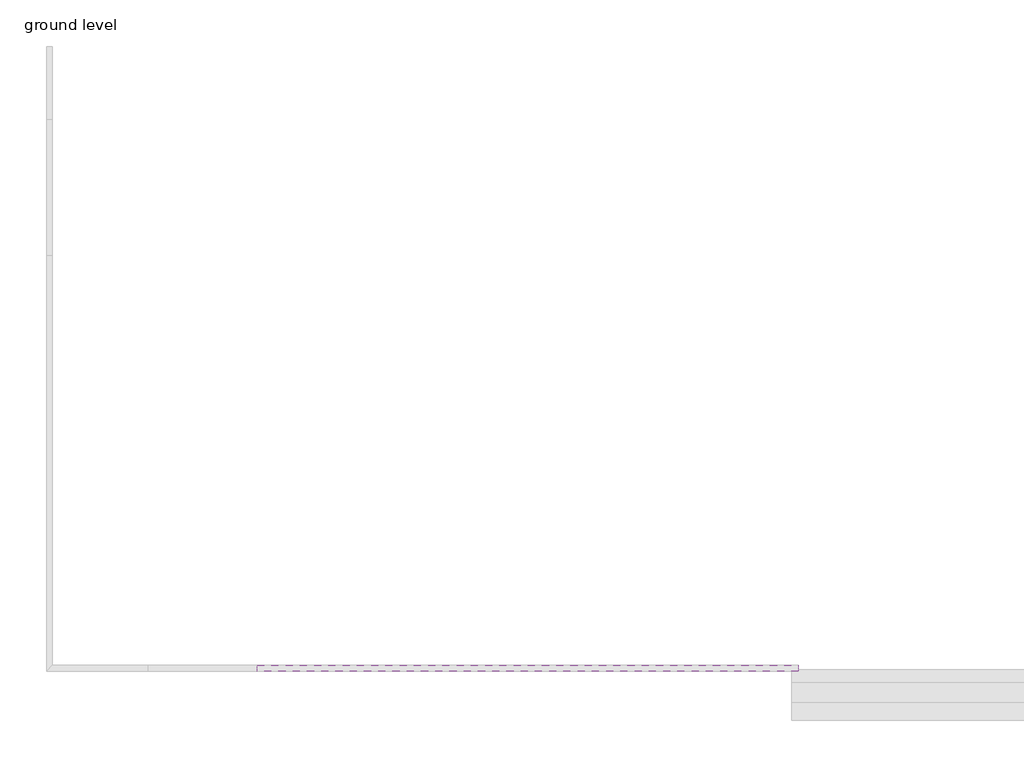
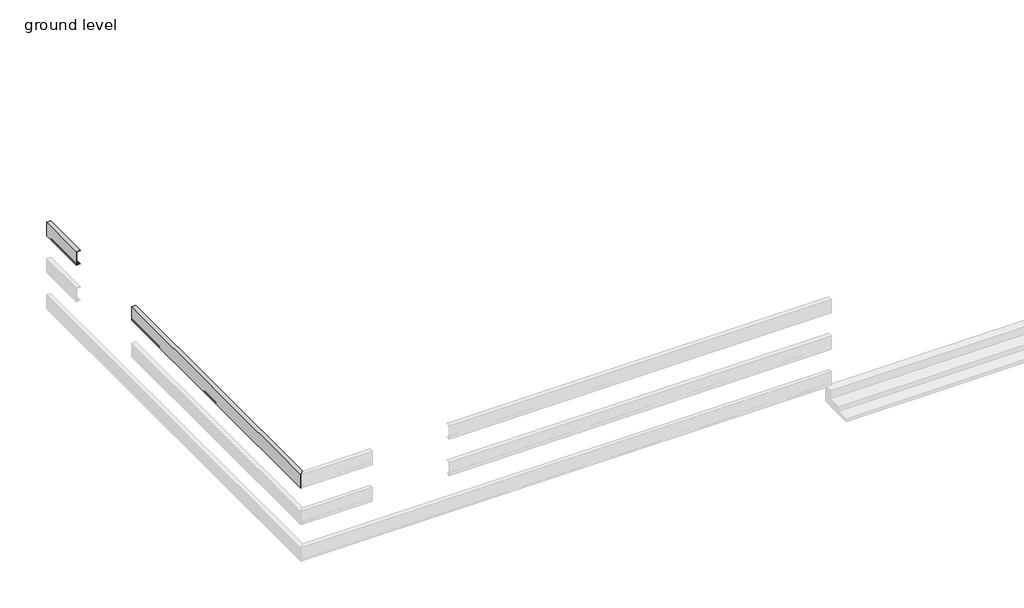
# One storey, part 2 of 3: 1 proxy.
"""IFC4 building model written with IfcOpenShell, lengths in millimetres."""

from ifc_helpers import new_model, si_unit, frame, origin, place, context, project, spatial, polyline, circle_curve, ellipse_curve, element, save
from ifc_brep_helpers import plane_surface, cylinder_surface, revolved_surface, advanced_brep

model = new_model("IFC4")

# Units and contexts
model_context = context("Model", 3, world=origin())
ifc_project = project(units=[si_unit("LENGTHUNIT", "METRE", prefix="MILLI")], contexts=[model_context])

# Site, building, storey
site = spatial("IfcSite", under=ifc_project)
building = spatial("IfcBuilding", under=site)
storey = spatial("IfcBuildingStorey", under=building, Name="ground level", Elevation=0.0)

# Proxy
placement = place(None, origin())
element("IfcBuildingElementProxy", 1, Name="Reveal", ObjectType="Reveal", at=placement, inside=storey, context=model_context, shape_type="AdvancedBrep", body=[
    advanced_brep(
    [(-10842.2672301, -7280.1146427, 1689.1), (-10842.2672301, -7216.8686427, 1689.1), (-10842.2672301, -7216.8686427, 1687.7203242), (-10842.2672301, -7221.2514519, 1682.5465897), (-10842.2672301, -7244.8721427, 1678.6098), (-10842.2672301, -7264.1100243, 1675.40348), (-10842.2672301, -7272.8756427, 1665.056011), (-10842.2672301, -7272.8756427, 1484.543989), (-10842.2672301, -7264.1100243, 1474.19652), (-10842.2672301, -7244.8721427, 1470.9902), (-10842.2672301, -7221.2514519, 1467.0534103), (-10842.2672301, -7216.8686427, 1461.8796758), (-10842.2672301, -7216.8686427, 1460.5), (-10842.2672301, -7280.1146427, 1460.5), (-4797.0672301, -7280.1146427, 1689.1), (-4797.0672301, -7280.1146427, 1460.5), (-4797.0672301, -7216.8686427, 1460.5), (-4797.0672301, -7216.8686427, 1461.8796758), (-4797.0672301, -7221.2514519, 1467.0534103), (-4797.0672301, -7244.8721427, 1470.9902), (-4797.0672301, -7264.1100243, 1474.19652), (-4797.0672301, -7272.8756427, 1484.543989), (-4797.0672301, -7272.8756427, 1665.056011), (-4797.0672301, -7264.1100243, 1675.40348), (-4797.0672301, -7244.8721427, 1678.6098), (-4797.0672301, -7221.2514519, 1682.5465897), (-4797.0672301, -7216.8686427, 1687.7203242), (-4797.0672301, -7216.8686427, 1689.1)],
    [
        (0, 1),
        (1, 2),
        (2, 3, circle_curve(frame((-10842.2672301, -7222.1137427, 1687.7203242), z_axis=(-1.0, 0.0, 0.0), x_axis=(0.0, 1.0, 0.0)), 5.2451)),
        (3, 4),
        (4, 5),
        (5, 6, circle_curve(frame((-10842.2672301, -7262.3854427, 1665.056011), z_axis=(1.0, 0.0, 0.0), x_axis=(0.0, 1.0, 0.0)), 10.4902)),
        (6, 7),
        (7, 8, circle_curve(frame((-10842.2672301, -7262.3854427, 1484.543989), z_axis=(1.0, 0.0, 0.0), x_axis=(0.0, 1.0, 0.0)), 10.4902)),
        (8, 9),
        (9, 10),
        (10, 11, circle_curve(frame((-10842.2672301, -7222.1137427, 1461.8796758), z_axis=(-1.0, 0.0, 0.0), x_axis=(0.0, 1.0, 0.0)), 5.2451)),
        (11, 12),
        (12, 13),
        (13, 0),
        (14, 15),
        (15, 16),
        (16, 17),
        (17, 18, circle_curve(frame((-4797.0672301, -7222.1137427, 1461.8796758), z_axis=(1.0, 0.0, 0.0), x_axis=(0.0, 1.0, 0.0)), 5.2451)),
        (18, 19),
        (19, 20),
        (20, 21, circle_curve(frame((-4797.0672301, -7262.3854427, 1484.543989), z_axis=(-1.0, 0.0, 0.0), x_axis=(0.0, 1.0, 0.0)), 10.4902)),
        (21, 22),
        (22, 23, circle_curve(frame((-4797.0672301, -7262.3854427, 1665.056011), z_axis=(-1.0, 0.0, 0.0), x_axis=(0.0, 1.0, 0.0)), 10.4902)),
        (23, 24),
        (24, 25),
        (25, 26, circle_curve(frame((-4797.0672301, -7222.1137427, 1687.7203242), z_axis=(1.0, 0.0, 0.0), x_axis=(0.0, 1.0, 0.0)), 5.2451)),
        (26, 27),
        (27, 14),
        (0, 14),
        (27, 1),
        (26, 2),
        (25, 3),
        (24, 4),
        (23, 5),
        (22, 6),
        (21, 7),
        (20, 8),
        (19, 9),
        (18, 10),
        (17, 11),
        (16, 12),
        (15, 13),
    ],
    [
        plane_surface(frame((-10842.2672301, -7036.6302427, 914.4), z_axis=(-1.0, 0.0, 0.0), x_axis=(0.0, -1.0, 0.0))),
        plane_surface(frame((-4797.0672301, -7265.2302427, 1450.6898298), z_axis=(1.0, 0.0, 0.0), x_axis=(0.0, 1.0, 0.0))),
        plane_surface(frame((-10842.2672301, -7280.1146427, 1689.1), z_axis=(0.0, 0.0, 1.0), x_axis=(1.0, 0.0, 0.0))),
        plane_surface(frame((-10842.2672301, -7216.8686427, 1689.1), z_axis=(0.0, 1.0, 0.0), x_axis=(1.0, 0.0, 0.0))),
        cylinder_surface(frame((-10842.2672301, -7222.1137427, 1687.7203242), z_axis=(-1.0, 0.0, 0.0), x_axis=(0.0, 1.0, 0.0)), 5.2451),
        plane_surface(frame((-10842.2672301, -7221.2514519, 1682.5465897), z_axis=(0.0, 0.16439930721687082, -0.9863938705135049), x_axis=(1.0, 0.0, 0.0))),
        plane_surface(frame((-10842.2672301, -7244.8721427, 1678.6098), z_axis=(0.0, 0.16439930721687146, -0.9863938705135048), x_axis=(1.0, 0.0, 0.0))),
        revolved_surface(polyline([(-4797.0672301, -7251.8952426999995, 1665.056011), (-10842.2672301, -7251.8952426999995, 1665.056011)]), (-10842.2672301, -7262.3854427, 1665.056011), (1.0, 0.0, 0.0)),
        plane_surface(frame((-10842.2672301, -7272.8756427, 1665.056011), z_axis=(0.0, 1.0, 0.0), x_axis=(1.0, 0.0, 0.0))),
        revolved_surface(polyline([(-4797.0672301, -7251.8952426999995, 1484.543989), (-10842.2672301, -7251.8952426999995, 1484.543989)]), (-10842.2672301, -7262.3854427, 1484.543989), (1.0, 0.0, 0.0)),
        plane_surface(frame((-10842.2672301, -7264.1100243, 1474.19652), z_axis=(0.0, 0.1643993072168769, 0.9863938705135039), x_axis=(1.0, 0.0, 0.0))),
        plane_surface(frame((-10842.2672301, -7244.8721427, 1470.9902), z_axis=(0.0, 0.16439930721687793, 0.9863938705135037), x_axis=(1.0, 0.0, 0.0))),
        cylinder_surface(frame((-10842.2672301, -7222.1137427, 1461.8796758), z_axis=(-1.0, 0.0, 0.0), x_axis=(0.0, 1.0, 0.0)), 5.2451),
        plane_surface(frame((-10842.2672301, -7216.8686427, 1461.8796758), z_axis=(0.0, 1.0, 0.0), x_axis=(1.0, 0.0, 0.0))),
        plane_surface(frame((-10842.2672301, -7216.8686427, 1460.5), z_axis=(0.0, 0.0, -1.0), x_axis=(1.0, 0.0, 0.0))),
        plane_surface(frame((-10842.2672301, -7280.1146427, 1460.5), z_axis=(0.0, -1.0, 0.0), x_axis=(1.0, 0.0, 0.0))),
    ],
    [
        (0, [[1, 2, 3, 4, 5, 6, 7, 8, 9, 10, 11, 12, 13, 14]]),
        (1, [[15, 16, 17, 18, 19, 20, 21, 22, 23, 24, 25, 26, 27, 28]]),
        (2, [[-1, 29, -28, 30]]),
        (3, [[-2, -30, -27, 31]]),
        (4, [[-3, -31, -26, 32]]),
        (5, [[-4, -32, -25, 33]]),
        (6, [[-5, -33, -24, 34]]),
        (7, [[-6, -34, -23, 35]]),
        (8, [[-7, -35, -22, 36]]),
        (9, [[-8, -36, -21, 37]]),
        (10, [[-9, -37, -20, 38]]),
        (11, [[-10, -38, -19, 39]]),
        (12, [[-11, -39, -18, 40]]),
        (13, [[-12, -40, -17, 41]]),
        (14, [[-13, -41, -16, 42]]),
        (15, [[-14, -42, -15, -29]]),
    ],
),
    advanced_brep(
    [(-13193.9516301, -7280.1146427, 1689.1), (-13130.7056301, -7216.8686427, 1689.1), (-13130.7056301, -7216.8686427, 1687.7203242), (-13135.0884393, -7221.2514519, 1682.5465897), (-13158.7091301, -7244.8721427, 1678.6098), (-13177.9470117, -7264.1100243, 1675.40348), (-13186.7126301, -7272.8756427, 1665.056011), (-13186.7126301, -7272.8756427, 1484.543989), (-13177.9470117, -7264.1100243, 1474.19652), (-13158.7091301, -7244.8721427, 1470.9902), (-13135.0884393, -7221.2514519, 1467.0534103), (-13130.7056301, -7216.8686427, 1461.8796758), (-13130.7056301, -7216.8686427, 1460.5), (-13193.9516301, -7280.1146427, 1460.5), (-12061.4672301, -7280.1146427, 1689.1), (-12061.4672301, -7280.1146427, 1460.5), (-12061.4672301, -7216.8686427, 1460.5), (-12061.4672301, -7216.8686427, 1461.8796758), (-12061.4672301, -7221.2514519, 1467.0534103), (-12061.4672301, -7244.8721427, 1470.9902), (-12061.4672301, -7264.1100243, 1474.19652), (-12061.4672301, -7272.8756427, 1484.543989), (-12061.4672301, -7272.8756427, 1665.056011), (-12061.4672301, -7264.1100243, 1675.40348), (-12061.4672301, -7244.8721427, 1678.6098), (-12061.4672301, -7221.2514519, 1682.5465897), (-12061.4672301, -7216.8686427, 1687.7203242), (-12061.4672301, -7216.8686427, 1689.1)],
    [
        (0, 1),
        (1, 2),
        (2, 3, ellipse_curve(frame((-13135.9507301, -7222.1137427, 1687.7203242), z_axis=(-0.7071067811865476, 0.7071067811865476, 0.0), x_axis=(-0.7071067811865475, -0.7071067811865476, 0.0)), 7.4176916, 5.2451)),
        (3, 4),
        (4, 5),
        (5, 6, ellipse_curve(frame((-13176.2224301, -7262.3854427, 1665.056011), z_axis=(0.7071067811865476, -0.7071067811865476, 0.0), x_axis=(0.7071067811865475, 0.7071067811865476, 0.0)), 14.8353831, 10.4902)),
        (6, 7),
        (7, 8, ellipse_curve(frame((-13176.2224301, -7262.3854427, 1484.543989), z_axis=(0.7071067811865476, -0.7071067811865476, 0.0), x_axis=(0.7071067811865475, 0.7071067811865476, 0.0)), 14.8353831, 10.4902)),
        (8, 9),
        (9, 10),
        (10, 11, ellipse_curve(frame((-13135.9507301, -7222.1137427, 1461.8796758), z_axis=(-0.7071067811865476, 0.7071067811865476, 0.0), x_axis=(-0.7071067811865475, -0.7071067811865476, 0.0)), 7.4176916, 5.2451)),
        (11, 12),
        (12, 13),
        (13, 0),
        (14, 15),
        (15, 16),
        (16, 17),
        (17, 18, circle_curve(frame((-12061.4672301, -7222.1137427, 1461.8796758), z_axis=(1.0, 0.0, 0.0), x_axis=(0.0, 1.0, 0.0)), 5.2451)),
        (18, 19),
        (19, 20),
        (20, 21, circle_curve(frame((-12061.4672301, -7262.3854427, 1484.543989), z_axis=(-1.0, 0.0, 0.0), x_axis=(0.0, 1.0, 0.0)), 10.4902)),
        (21, 22),
        (22, 23, circle_curve(frame((-12061.4672301, -7262.3854427, 1665.056011), z_axis=(-1.0, 0.0, 0.0), x_axis=(0.0, 1.0, 0.0)), 10.4902)),
        (23, 24),
        (24, 25),
        (25, 26, circle_curve(frame((-12061.4672301, -7222.1137427, 1687.7203242), z_axis=(1.0, 0.0, 0.0), x_axis=(0.0, 1.0, 0.0)), 5.2451)),
        (26, 27),
        (27, 14),
        (0, 14),
        (27, 1),
        (26, 2),
        (25, 3),
        (24, 4),
        (23, 5),
        (22, 6),
        (21, 7),
        (20, 8),
        (19, 9),
        (18, 10),
        (17, 11),
        (16, 12),
        (15, 13),
    ],
    [
        plane_surface(frame((-13179.0672301, -7265.2302427, 1270.0), z_axis=(-0.7071067811865476, 0.7071067811865476, 0.0), x_axis=(0.7071067811865476, 0.7071067811865476, 0.0))),
        plane_surface(frame((-12061.4672301, -7036.6302427, 2184.4), z_axis=(1.0, 0.0, 0.0), x_axis=(0.0, -1.0, 0.0))),
        plane_surface(frame((-13193.9516301, -7280.1146427, 1689.1), z_axis=(0.0, 0.0, 1.0), x_axis=(1.0, 0.0, 0.0))),
        plane_surface(frame((-13130.7056301, -7216.8686427, 1689.1), z_axis=(0.0, 1.0, 0.0), x_axis=(1.0, 0.0, 0.0))),
        cylinder_surface(frame((-13179.0672301, -7222.1137427, 1687.7203242), z_axis=(-1.0, 0.0, 0.0), x_axis=(0.0, 1.0, 0.0)), 5.2451),
        plane_surface(frame((-13135.0884393, -7221.2514519, 1682.5465897), z_axis=(0.0, 0.16439930721687082, -0.9863938705135049), x_axis=(1.0, 0.0, 0.0))),
        plane_surface(frame((-13158.7091301, -7244.8721427, 1678.6098), z_axis=(0.0, 0.16439930721687146, -0.9863938705135048), x_axis=(1.0, 0.0, 0.0))),
        revolved_surface(polyline([(-12061.4672301, -7251.8952426999995, 1665.056011), (-13186.7126301, -7251.8952426999995, 1665.056011)]), (-13179.0672301, -7262.3854427, 1665.056011), (1.0, 0.0, 0.0)),
        plane_surface(frame((-13186.7126301, -7272.8756427, 1665.056011), z_axis=(0.0, 1.0, 0.0), x_axis=(1.0, 0.0, 0.0))),
        revolved_surface(polyline([(-12061.4672301, -7251.8952426999995, 1484.543989), (-13186.7126301, -7251.8952426999995, 1484.543989)]), (-13179.0672301, -7262.3854427, 1484.543989), (1.0, 0.0, 0.0)),
        plane_surface(frame((-13177.9470117, -7264.1100243, 1474.19652), z_axis=(0.0, 0.1643993072168769, 0.9863938705135039), x_axis=(1.0, 0.0, 0.0))),
        plane_surface(frame((-13158.7091301, -7244.8721427, 1470.9902), z_axis=(0.0, 0.16439930721687793, 0.9863938705135037), x_axis=(1.0, 0.0, 0.0))),
        cylinder_surface(frame((-13179.0672301, -7222.1137427, 1461.8796758), z_axis=(-1.0, 0.0, 0.0), x_axis=(0.0, 1.0, 0.0)), 5.2451),
        plane_surface(frame((-13130.7056301, -7216.8686427, 1461.8796758), z_axis=(0.0, 1.0, 0.0), x_axis=(1.0, 0.0, 0.0))),
        plane_surface(frame((-13130.7056301, -7216.8686427, 1460.5), z_axis=(0.0, 0.0, -1.0), x_axis=(1.0, 0.0, 0.0))),
        plane_surface(frame((-13193.9516301, -7280.1146427, 1460.5), z_axis=(0.0, -1.0, 0.0), x_axis=(1.0, 0.0, 0.0))),
    ],
    [
        (0, [[1, 2, 3, 4, 5, 6, 7, 8, 9, 10, 11, 12, 13, 14]]),
        (1, [[15, 16, 17, 18, 19, 20, 21, 22, 23, 24, 25, 26, 27, 28]]),
        (2, [[-1, 29, -28, 30]]),
        (3, [[-2, -30, -27, 31]]),
        (4, [[-3, -31, -26, 32]]),
        (5, [[-4, -32, -25, 33]]),
        (6, [[-5, -33, -24, 34]]),
        (7, [[-6, -34, -23, 35]]),
        (8, [[-7, -35, -22, 36]]),
        (9, [[-8, -36, -21, 37]]),
        (10, [[-9, -37, -20, 38]]),
        (11, [[-10, -38, -19, 39]]),
        (12, [[-11, -39, -18, 40]]),
        (13, [[-12, -40, -17, 41]]),
        (14, [[-13, -41, -16, 42]]),
        (15, [[-14, -42, -15, -29]]),
    ],
),
    advanced_brep(
    [(-13193.9516301, -2642.4302427, 1689.1), (-13130.7056301, -2642.4302427, 1689.1), (-13130.7056301, -2642.4302427, 1687.7203242), (-13135.0884393, -2642.4302427, 1682.5465897), (-13158.7091301, -2642.4302427, 1678.6098), (-13177.9470117, -2642.4302427, 1675.40348), (-13186.7126301, -2642.4302427, 1665.056011), (-13186.7126301, -2642.4302427, 1484.543989), (-13177.9470117, -2642.4302427, 1474.19652), (-13158.7091301, -2642.4302427, 1470.9902), (-13135.0884393, -2642.4302427, 1467.0534103), (-13130.7056301, -2642.4302427, 1461.8796758), (-13130.7056301, -2642.4302427, 1460.5), (-13193.9516301, -2642.4302427, 1460.5), (-13193.9516301, -7280.1146427, 1689.1), (-13193.9516301, -7280.1146427, 1460.5), (-13130.7056301, -7216.8686427, 1460.5), (-13130.7056301, -7216.8686427, 1461.8796758), (-13135.0884393, -7221.2514519, 1467.0534103), (-13158.7091301, -7244.8721427, 1470.9902), (-13177.9470117, -7264.1100243, 1474.19652), (-13186.7126301, -7272.8756427, 1484.543989), (-13186.7126301, -7272.8756427, 1665.056011), (-13177.9470117, -7264.1100243, 1675.40348), (-13158.7091301, -7244.8721427, 1678.6098), (-13135.0884393, -7221.2514519, 1682.5465897), (-13130.7056301, -7216.8686427, 1687.7203242), (-13130.7056301, -7216.8686427, 1689.1)],
    [
        (0, 1),
        (1, 2),
        (2, 3, circle_curve(frame((-13135.9507301, -2642.4302427, 1687.7203242), z_axis=(0.0, 1.0, 0.0), x_axis=(1.0, 0.0, 0.0)), 5.2451)),
        (3, 4),
        (4, 5),
        (5, 6, circle_curve(frame((-13176.2224301, -2642.4302427, 1665.056011), z_axis=(0.0, -1.0, 0.0), x_axis=(1.0, 0.0, 0.0)), 10.4902)),
        (6, 7),
        (7, 8, circle_curve(frame((-13176.2224301, -2642.4302427, 1484.543989), z_axis=(0.0, -1.0, 0.0), x_axis=(1.0, 0.0, 0.0)), 10.4902)),
        (8, 9),
        (9, 10),
        (10, 11, circle_curve(frame((-13135.9507301, -2642.4302427, 1461.8796758), z_axis=(0.0, 1.0, 0.0), x_axis=(1.0, 0.0, 0.0)), 5.2451)),
        (11, 12),
        (12, 13),
        (13, 0),
        (14, 15),
        (15, 16),
        (16, 17),
        (17, 18, ellipse_curve(frame((-13135.9507301, -7222.1137427, 1461.8796758), z_axis=(0.7071067811865476, -0.7071067811865476, 0.0), x_axis=(0.7071067811865477, 0.7071067811865474, 0.0)), 7.4176916, 5.2451)),
        (18, 19),
        (19, 20),
        (20, 21, ellipse_curve(frame((-13176.2224301, -7262.3854427, 1484.543989), z_axis=(-0.7071067811865476, 0.7071067811865476, 0.0), x_axis=(-0.7071067811865477, -0.7071067811865474, 0.0)), 14.8353831, 10.4902)),
        (21, 22),
        (22, 23, ellipse_curve(frame((-13176.2224301, -7262.3854427, 1665.056011), z_axis=(-0.7071067811865476, 0.7071067811865476, 0.0), x_axis=(-0.7071067811865477, -0.7071067811865474, 0.0)), 14.8353831, 10.4902)),
        (23, 24),
        (24, 25),
        (25, 26, ellipse_curve(frame((-13135.9507301, -7222.1137427, 1687.7203242), z_axis=(0.7071067811865476, -0.7071067811865476, 0.0), x_axis=(0.7071067811865477, 0.7071067811865474, 0.0)), 7.4176916, 5.2451)),
        (26, 27),
        (27, 14),
        (0, 14),
        (27, 1),
        (26, 2),
        (25, 3),
        (24, 4),
        (23, 5),
        (22, 6),
        (21, 7),
        (20, 8),
        (19, 9),
        (18, 10),
        (17, 11),
        (16, 12),
        (15, 13),
    ],
    [
        plane_surface(frame((-12950.4672301, -2642.4302427, 914.4), z_axis=(0.0, 1.0, 0.0), x_axis=(-1.0, 0.0, 0.0))),
        plane_surface(frame((-13179.0672301, -7265.2302427, 1270.0), z_axis=(0.7071067811865476, -0.7071067811865476, 0.0), x_axis=(0.7071067811865476, 0.7071067811865476, 0.0))),
        plane_surface(frame((-13193.9516301, -2642.4302427, 1689.1), z_axis=(0.0, 0.0, 1.0), x_axis=(0.0, -1.0, 0.0))),
        plane_surface(frame((-13130.7056301, -2642.4302427, 1689.1), z_axis=(1.0, 0.0, 0.0), x_axis=(0.0, -1.0, 0.0))),
        cylinder_surface(frame((-13135.9507301, -2642.4302427, 1687.7203242), z_axis=(0.0, 1.0, 0.0), x_axis=(1.0, 0.0, 0.0)), 5.2451),
        plane_surface(frame((-13135.0884393, -2642.4302427, 1682.5465897), z_axis=(0.16439930721687082, 0.0, -0.9863938705135049), x_axis=(0.0, -1.0, 0.0))),
        plane_surface(frame((-13158.7091301, -2642.4302427, 1678.6098), z_axis=(0.16439930721687146, 0.0, -0.9863938705135048), x_axis=(0.0, -1.0, 0.0))),
        revolved_surface(polyline([(-13165.7322301, -7272.875642700001, 1665.056011), (-13165.7322301, -2642.4302427, 1665.056011)]), (-13176.2224301, -2642.4302427, 1665.056011), (0.0, -1.0, 0.0)),
        plane_surface(frame((-13186.7126301, -2642.4302427, 1665.056011), z_axis=(1.0, 0.0, 0.0), x_axis=(0.0, -1.0, 0.0))),
        revolved_surface(polyline([(-13165.7322301, -7272.875642700001, 1484.543989), (-13165.7322301, -2642.4302427, 1484.543989)]), (-13176.2224301, -2642.4302427, 1484.543989), (0.0, -1.0, 0.0)),
        plane_surface(frame((-13177.9470117, -2642.4302427, 1474.19652), z_axis=(0.1643993072168769, 0.0, 0.9863938705135039), x_axis=(0.0, -1.0, 0.0))),
        plane_surface(frame((-13158.7091301, -2642.4302427, 1470.9902), z_axis=(0.16439930721687793, 0.0, 0.9863938705135037), x_axis=(0.0, -1.0, 0.0))),
        cylinder_surface(frame((-13135.9507301, -2642.4302427, 1461.8796758), z_axis=(0.0, 1.0, 0.0), x_axis=(1.0, 0.0, 0.0)), 5.2451),
        plane_surface(frame((-13130.7056301, -2642.4302427, 1461.8796758), z_axis=(1.0, 0.0, 0.0), x_axis=(0.0, -1.0, 0.0))),
        plane_surface(frame((-13130.7056301, -2642.4302427, 1460.5), z_axis=(0.0, 0.0, -1.0), x_axis=(0.0, -1.0, 0.0))),
        plane_surface(frame((-13193.9516301, -2642.4302427, 1460.5), z_axis=(-1.0, 0.0, 0.0), x_axis=(0.0, -1.0, 0.0))),
    ],
    [
        (0, [[1, 2, 3, 4, 5, 6, 7, 8, 9, 10, 11, 12, 13, 14]]),
        (1, [[15, 16, 17, 18, 19, 20, 21, 22, 23, 24, 25, 26, 27, 28]]),
        (2, [[-1, 29, -28, 30]]),
        (3, [[-2, -30, -27, 31]]),
        (4, [[-3, -31, -26, 32]]),
        (5, [[-4, -32, -25, 33]]),
        (6, [[-5, -33, -24, 34]]),
        (7, [[-6, -34, -23, 35]]),
        (8, [[-7, -35, -22, 36]]),
        (9, [[-8, -36, -21, 37]]),
        (10, [[-9, -37, -20, 38]]),
        (11, [[-10, -38, -19, 39]]),
        (12, [[-11, -39, -18, 40]]),
        (13, [[-12, -40, -17, 41]]),
        (14, [[-13, -41, -16, 42]]),
        (15, [[-14, -42, -15, -29]]),
    ],
),
    advanced_brep(
    [(-13193.9516301, -305.6302427, 1689.1), (-13130.7056301, -305.6302427, 1689.1), (-13130.7056301, -305.6302427, 1687.7203242), (-13135.0884393, -305.6302427, 1682.5465897), (-13158.7091301, -305.6302427, 1678.6098), (-13177.9470117, -305.6302427, 1675.40348), (-13186.7126301, -305.6302427, 1665.056011), (-13186.7126301, -305.6302427, 1484.543989), (-13177.9470117, -305.6302427, 1474.19652), (-13158.7091301, -305.6302427, 1470.9902), (-13135.0884393, -305.6302427, 1467.0534103), (-13130.7056301, -305.6302427, 1461.8796758), (-13130.7056301, -305.6302427, 1460.5), (-13193.9516301, -305.6302427, 1460.5), (-13193.9516301, -1118.4302427, 1689.1), (-13193.9516301, -1118.4302427, 1460.5), (-13130.7056301, -1118.4302427, 1460.5), (-13130.7056301, -1118.4302427, 1461.8796758), (-13135.0884393, -1118.4302427, 1467.0534103), (-13158.7091301, -1118.4302427, 1470.9902), (-13177.9470117, -1118.4302427, 1474.19652), (-13186.7126301, -1118.4302427, 1484.543989), (-13186.7126301, -1118.4302427, 1665.056011), (-13177.9470117, -1118.4302427, 1675.40348), (-13158.7091301, -1118.4302427, 1678.6098), (-13135.0884393, -1118.4302427, 1682.5465897), (-13130.7056301, -1118.4302427, 1687.7203242), (-13130.7056301, -1118.4302427, 1689.1)],
    [
        (0, 1),
        (1, 2),
        (2, 3, circle_curve(frame((-13135.9507301, -305.6302427, 1687.7203242), z_axis=(0.0, 1.0, 0.0), x_axis=(1.0, 0.0, 0.0)), 5.2451)),
        (3, 4),
        (4, 5),
        (5, 6, circle_curve(frame((-13176.2224301, -305.6302427, 1665.056011), z_axis=(0.0, -1.0, 0.0), x_axis=(1.0, 0.0, 0.0)), 10.4902)),
        (6, 7),
        (7, 8, circle_curve(frame((-13176.2224301, -305.6302427, 1484.543989), z_axis=(0.0, -1.0, 0.0), x_axis=(1.0, 0.0, 0.0)), 10.4902)),
        (8, 9),
        (9, 10),
        (10, 11, circle_curve(frame((-13135.9507301, -305.6302427, 1461.8796758), z_axis=(0.0, 1.0, 0.0), x_axis=(1.0, 0.0, 0.0)), 5.2451)),
        (11, 12),
        (12, 13),
        (13, 0),
        (14, 15),
        (15, 16),
        (16, 17),
        (17, 18, circle_curve(frame((-13135.9507301, -1118.4302427, 1461.8796758), z_axis=(0.0, -1.0, 0.0), x_axis=(1.0, 0.0, 0.0)), 5.2451)),
        (18, 19),
        (19, 20),
        (20, 21, circle_curve(frame((-13176.2224301, -1118.4302427, 1484.543989), z_axis=(0.0, 1.0, 0.0), x_axis=(1.0, 0.0, 0.0)), 10.4902)),
        (21, 22),
        (22, 23, circle_curve(frame((-13176.2224301, -1118.4302427, 1665.056011), z_axis=(0.0, 1.0, 0.0), x_axis=(1.0, 0.0, 0.0)), 10.4902)),
        (23, 24),
        (24, 25),
        (25, 26, circle_curve(frame((-13135.9507301, -1118.4302427, 1687.7203242), z_axis=(0.0, -1.0, 0.0), x_axis=(1.0, 0.0, 0.0)), 5.2451)),
        (26, 27),
        (27, 14),
        (0, 14),
        (27, 1),
        (26, 2),
        (25, 3),
        (24, 4),
        (23, 5),
        (22, 6),
        (21, 7),
        (20, 8),
        (19, 9),
        (18, 10),
        (17, 11),
        (16, 12),
        (15, 13),
    ],
    [
        plane_surface(frame((-12942.6830845, -305.6302427, 304.8), z_axis=(0.0, 1.0, 0.0), x_axis=(-1.0, 0.0, 0.0))),
        plane_surface(frame((-12950.4672301, -1118.4302427, 2489.2), z_axis=(0.0, -1.0, 0.0), x_axis=(-1.0, 0.0, 0.0))),
        plane_surface(frame((-13193.9516301, -305.6302427, 1689.1), z_axis=(0.0, 0.0, 1.0), x_axis=(0.0, -1.0, 0.0))),
        plane_surface(frame((-13130.7056301, -305.6302427, 1689.1), z_axis=(1.0, 0.0, 0.0), x_axis=(0.0, -1.0, 0.0))),
        cylinder_surface(frame((-13135.9507301, -305.6302427, 1687.7203242), z_axis=(0.0, 1.0, 0.0), x_axis=(1.0, 0.0, 0.0)), 5.2451),
        plane_surface(frame((-13135.0884393, -305.6302427, 1682.5465897), z_axis=(0.16439930721687082, 0.0, -0.9863938705135049), x_axis=(0.0, -1.0, 0.0))),
        plane_surface(frame((-13158.7091301, -305.6302427, 1678.6098), z_axis=(0.16439930721687146, 0.0, -0.9863938705135048), x_axis=(0.0, -1.0, 0.0))),
        revolved_surface(polyline([(-13165.7322301, -1118.4302427, 1665.056011), (-13165.7322301, -305.6302427, 1665.056011)]), (-13176.2224301, -305.6302427, 1665.056011), (0.0, -1.0, 0.0)),
        plane_surface(frame((-13186.7126301, -305.6302427, 1665.056011), z_axis=(1.0, 0.0, 0.0), x_axis=(0.0, -1.0, 0.0))),
        revolved_surface(polyline([(-13165.7322301, -1118.4302427, 1484.543989), (-13165.7322301, -305.6302427, 1484.543989)]), (-13176.2224301, -305.6302427, 1484.543989), (0.0, -1.0, 0.0)),
        plane_surface(frame((-13177.9470117, -305.6302427, 1474.19652), z_axis=(0.1643993072168769, 0.0, 0.9863938705135039), x_axis=(0.0, -1.0, 0.0))),
        plane_surface(frame((-13158.7091301, -305.6302427, 1470.9902), z_axis=(0.16439930721687793, 0.0, 0.9863938705135037), x_axis=(0.0, -1.0, 0.0))),
        cylinder_surface(frame((-13135.9507301, -305.6302427, 1461.8796758), z_axis=(0.0, 1.0, 0.0), x_axis=(1.0, 0.0, 0.0)), 5.2451),
        plane_surface(frame((-13130.7056301, -305.6302427, 1461.8796758), z_axis=(1.0, 0.0, 0.0), x_axis=(0.0, -1.0, 0.0))),
        plane_surface(frame((-13130.7056301, -305.6302427, 1460.5), z_axis=(0.0, 0.0, -1.0), x_axis=(0.0, -1.0, 0.0))),
        plane_surface(frame((-13193.9516301, -305.6302427, 1460.5), z_axis=(-1.0, 0.0, 0.0), x_axis=(0.0, -1.0, 0.0))),
    ],
    [
        (0, [[1, 2, 3, 4, 5, 6, 7, 8, 9, 10, 11, 12, 13, 14]]),
        (1, [[15, 16, 17, 18, 19, 20, 21, 22, 23, 24, 25, 26, 27, 28]]),
        (2, [[-1, 29, -28, 30]]),
        (3, [[-2, -30, -27, 31]]),
        (4, [[-3, -31, -26, 32]]),
        (5, [[-4, -32, -25, 33]]),
        (6, [[-5, -33, -24, 34]]),
        (7, [[-6, -34, -23, 35]]),
        (8, [[-7, -35, -22, 36]]),
        (9, [[-8, -36, -21, 37]]),
        (10, [[-9, -37, -20, 38]]),
        (11, [[-10, -38, -19, 39]]),
        (12, [[-11, -39, -18, 40]]),
        (13, [[-12, -40, -17, 41]]),
        (14, [[-13, -41, -16, 42]]),
        (15, [[-14, -42, -15, -29]]),
    ],
),
])

save(model, "model.ifc")
